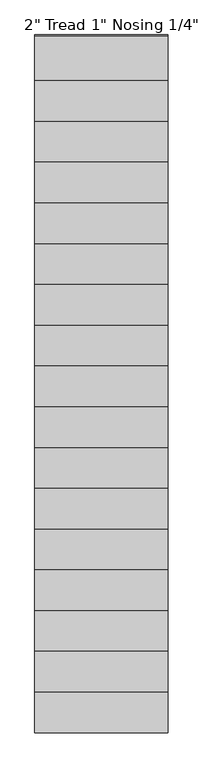
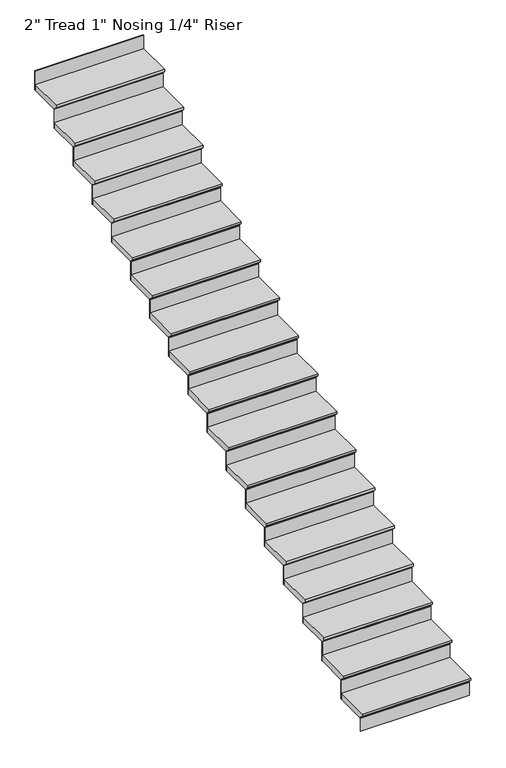
"""IFC4 building model written with IfcOpenShell, lengths in millimetres: stair flight geometry."""

from ifc_helpers import new_model, si_unit, frame, origin, place, context, project, spatial, polyline, outline, extrude, source, transform, mapped, element, save


def stair_flight_6f7ba89f(model_context):
    return source(origin(), model_context, "Body", "SweptSolid", [
        extrude(outline(polyline([(2020.7325341, 3522.1333333), (2325.5325341, 3522.1333333), (2325.5325341, 3471.3333333), (2046.1325341, 3471.3333333), (2046.1325341, 3477.6833333), (2020.7325341, 3503.0833333), (2020.7325341, 3522.1333333)])), frame((-5721.5875748, 0.0, 0.0), z_axis=(1.0, 0.0, 0.0), x_axis=(0.0, 1.0, 0.0)), (0.0, 0.0, 1.0), 914.4),
        extrude(outline(polyline([(-4807.1875748, 2052.4825341), (-4807.1875748, 2046.1325341), (-5721.5875748, 2046.1325341), (-5721.5875748, 2052.4825341), (-4807.1875748, 2052.4825341)])), frame((0.0, 0.0, 3352.8), z_axis=(0.0, 0.0, 1.0), x_axis=(1.0, 0.0, 0.0)), (0.0, 0.0, 1.0), 118.5333333),
        extrude(outline(polyline([(-4807.1875748, 2331.8825341), (-4807.1875748, 2325.5325341), (-5721.5875748, 2325.5325341), (-5721.5875748, 2331.8825341), (-4807.1875748, 2331.8825341)])), frame((0.0, 0.0, 3471.3333333), z_axis=(0.0, 0.0, 1.0), x_axis=(1.0, 0.0, 0.0)), (0.0, 0.0, 1.0), 169.3333333),
        extrude(outline(polyline([(2300.1325341, 3691.4666667), (2604.9325341, 3691.4666667), (2604.9325341, 3640.6666667), (2325.5325341, 3640.6666667), (2325.5325341, 3647.0166667), (2300.1325341, 3672.4166667), (2300.1325341, 3691.4666667)])), frame((-5721.5875748, 0.0, 0.0), z_axis=(1.0, 0.0, 0.0), x_axis=(0.0, 1.0, 0.0)), (0.0, 0.0, 1.0), 914.4),
        extrude(outline(polyline([(-4807.1875748, 2611.2825341), (-4807.1875748, 2604.9325341), (-5721.5875748, 2604.9325341), (-5721.5875748, 2611.2825341), (-4807.1875748, 2611.2825341)])), frame((0.0, 0.0, 3640.6666667), z_axis=(0.0, 0.0, 1.0), x_axis=(1.0, 0.0, 0.0)), (0.0, 0.0, 1.0), 169.3333333),
        extrude(outline(polyline([(2579.5325341, 3860.8), (2884.3325341, 3860.8), (2884.3325341, 3810.0), (2604.9325341, 3810.0), (2604.9325341, 3816.35), (2579.5325341, 3841.75), (2579.5325341, 3860.8)])), frame((-5721.5875748, 0.0, 0.0), z_axis=(1.0, 0.0, 0.0), x_axis=(0.0, 1.0, 0.0)), (0.0, 0.0, 1.0), 914.4),
        extrude(outline(polyline([(-4807.1875748, 2890.6825341), (-4807.1875748, 2884.3325341), (-5721.5875748, 2884.3325341), (-5721.5875748, 2890.6825341), (-4807.1875748, 2890.6825341)])), frame((0.0, 0.0, 3810.0), z_axis=(0.0, 0.0, 1.0), x_axis=(1.0, 0.0, 0.0)), (0.0, 0.0, 1.0), 169.3333333),
        extrude(outline(polyline([(2858.9325341, 4030.1333333), (3163.7325341, 4030.1333333), (3163.7325341, 3979.3333333), (2884.3325341, 3979.3333333), (2884.3325341, 3985.6833333), (2858.9325341, 4011.0833333), (2858.9325341, 4030.1333333)])), frame((-5721.5875748, 0.0, 0.0), z_axis=(1.0, 0.0, 0.0), x_axis=(0.0, 1.0, 0.0)), (0.0, 0.0, 1.0), 914.4),
        extrude(outline(polyline([(-4807.1875748, 3170.0825341), (-4807.1875748, 3163.7325341), (-5721.5875748, 3163.7325341), (-5721.5875748, 3170.0825341), (-4807.1875748, 3170.0825341)])), frame((0.0, 0.0, 3979.3333333), z_axis=(0.0, 0.0, 1.0), x_axis=(1.0, 0.0, 0.0)), (0.0, 0.0, 1.0), 169.3333333),
        extrude(outline(polyline([(3138.3325341, 4199.4666667), (3443.1325341, 4199.4666667), (3443.1325341, 4148.6666667), (3163.7325341, 4148.6666667), (3163.7325341, 4155.0166667), (3138.3325341, 4180.4166667), (3138.3325341, 4199.4666667)])), frame((-5721.5875748, 0.0, 0.0), z_axis=(1.0, 0.0, 0.0), x_axis=(0.0, 1.0, 0.0)), (0.0, 0.0, 1.0), 914.4),
        extrude(outline(polyline([(-4807.1875748, 3449.4825341), (-4807.1875748, 3443.1325341), (-5721.5875748, 3443.1325341), (-5721.5875748, 3449.4825341), (-4807.1875748, 3449.4825341)])), frame((0.0, 0.0, 4148.6666667), z_axis=(0.0, 0.0, 1.0), x_axis=(1.0, 0.0, 0.0)), (0.0, 0.0, 1.0), 169.3333333),
        extrude(outline(polyline([(3417.7325341, 4368.8), (3722.5325341, 4368.8), (3722.5325341, 4318.0), (3443.1325341, 4318.0), (3443.1325341, 4324.35), (3417.7325341, 4349.75), (3417.7325341, 4368.8)])), frame((-5721.5875748, 0.0, 0.0), z_axis=(1.0, 0.0, 0.0), x_axis=(0.0, 1.0, 0.0)), (0.0, 0.0, 1.0), 914.4),
        extrude(outline(polyline([(-4807.1875748, 3728.8825341), (-4807.1875748, 3722.5325341), (-5721.5875748, 3722.5325341), (-5721.5875748, 3728.8825341), (-4807.1875748, 3728.8825341)])), frame((0.0, 0.0, 4318.0), z_axis=(0.0, 0.0, 1.0), x_axis=(1.0, 0.0, 0.0)), (0.0, 0.0, 1.0), 169.3333333),
        extrude(outline(polyline([(3697.1325341, 4538.1333333), (4001.9325341, 4538.1333333), (4001.9325341, 4487.3333333), (3722.5325341, 4487.3333333), (3722.5325341, 4493.6833333), (3697.1325341, 4519.0833333), (3697.1325341, 4538.1333333)])), frame((-5721.5875748, 0.0, 0.0), z_axis=(1.0, 0.0, 0.0), x_axis=(0.0, 1.0, 0.0)), (0.0, 0.0, 1.0), 914.4),
        extrude(outline(polyline([(-4807.1875748, 4008.2825341), (-4807.1875748, 4001.9325341), (-5721.5875748, 4001.9325341), (-5721.5875748, 4008.2825341), (-4807.1875748, 4008.2825341)])), frame((0.0, 0.0, 4487.3333333), z_axis=(0.0, 0.0, 1.0), x_axis=(1.0, 0.0, 0.0)), (0.0, 0.0, 1.0), 169.3333333),
        extrude(outline(polyline([(3976.5325341, 4707.4666667), (4281.3325341, 4707.4666667), (4281.3325341, 4656.6666667), (4001.9325341, 4656.6666667), (4001.9325341, 4663.0166667), (3976.5325341, 4688.4166667), (3976.5325341, 4707.4666667)])), frame((-5721.5875748, 0.0, 0.0), z_axis=(1.0, 0.0, 0.0), x_axis=(0.0, 1.0, 0.0)), (0.0, 0.0, 1.0), 914.4),
        extrude(outline(polyline([(-4807.1875748, 4287.6825341), (-4807.1875748, 4281.3325341), (-5721.5875748, 4281.3325341), (-5721.5875748, 4287.6825341), (-4807.1875748, 4287.6825341)])), frame((0.0, 0.0, 4656.6666667), z_axis=(0.0, 0.0, 1.0), x_axis=(1.0, 0.0, 0.0)), (0.0, 0.0, 1.0), 169.3333333),
        extrude(outline(polyline([(4255.9325341, 4876.8), (4560.7325341, 4876.8), (4560.7325341, 4826.0), (4281.3325341, 4826.0), (4281.3325341, 4832.35), (4255.9325341, 4857.75), (4255.9325341, 4876.8)])), frame((-5721.5875748, 0.0, 0.0), z_axis=(1.0, 0.0, 0.0), x_axis=(0.0, 1.0, 0.0)), (0.0, 0.0, 1.0), 914.4),
        extrude(outline(polyline([(-4807.1875748, 4567.0825341), (-4807.1875748, 4560.7325341), (-5721.5875748, 4560.7325341), (-5721.5875748, 4567.0825341), (-4807.1875748, 4567.0825341)])), frame((0.0, 0.0, 4826.0), z_axis=(0.0, 0.0, 1.0), x_axis=(1.0, 0.0, 0.0)), (0.0, 0.0, 1.0), 169.3333333),
        extrude(outline(polyline([(4535.3325341, 5046.1333333), (4840.1325341, 5046.1333333), (4840.1325341, 4995.3333333), (4560.7325341, 4995.3333333), (4560.7325341, 5001.6833333), (4535.3325341, 5027.0833333), (4535.3325341, 5046.1333333)])), frame((-5721.5875748, 0.0, 0.0), z_axis=(1.0, 0.0, 0.0), x_axis=(0.0, 1.0, 0.0)), (0.0, 0.0, 1.0), 914.4),
        extrude(outline(polyline([(-4807.1875748, 4846.4825341), (-4807.1875748, 4840.1325341), (-5721.5875748, 4840.1325341), (-5721.5875748, 4846.4825341), (-4807.1875748, 4846.4825341)])), frame((0.0, 0.0, 4995.3333333), z_axis=(0.0, 0.0, 1.0), x_axis=(1.0, 0.0, 0.0)), (0.0, 0.0, 1.0), 169.3333333),
        extrude(outline(polyline([(4814.7325341, 5215.4666667), (5119.5325341, 5215.4666667), (5119.5325341, 5164.6666667), (4840.1325341, 5164.6666667), (4840.1325341, 5171.0166667), (4814.7325341, 5196.4166667), (4814.7325341, 5215.4666667)])), frame((-5721.5875748, 0.0, 0.0), z_axis=(1.0, 0.0, 0.0), x_axis=(0.0, 1.0, 0.0)), (0.0, 0.0, 1.0), 914.4),
        extrude(outline(polyline([(-4807.1875748, 5125.8825341), (-4807.1875748, 5119.5325341), (-5721.5875748, 5119.5325341), (-5721.5875748, 5125.8825341), (-4807.1875748, 5125.8825341)])), frame((0.0, 0.0, 5164.6666667), z_axis=(0.0, 0.0, 1.0), x_axis=(1.0, 0.0, 0.0)), (0.0, 0.0, 1.0), 169.3333333),
        extrude(outline(polyline([(5094.1325341, 5384.8), (5398.9325341, 5384.8), (5398.9325341, 5334.0), (5119.5325341, 5334.0), (5119.5325341, 5340.35), (5094.1325341, 5365.75), (5094.1325341, 5384.8)])), frame((-5721.5875748, 0.0, 0.0), z_axis=(1.0, 0.0, 0.0), x_axis=(0.0, 1.0, 0.0)), (0.0, 0.0, 1.0), 914.4),
        extrude(outline(polyline([(-4807.1875748, 5405.2825341), (-4807.1875748, 5398.9325341), (-5721.5875748, 5398.9325341), (-5721.5875748, 5405.2825341), (-4807.1875748, 5405.2825341)])), frame((0.0, 0.0, 5334.0), z_axis=(0.0, 0.0, 1.0), x_axis=(1.0, 0.0, 0.0)), (0.0, 0.0, 1.0), 169.3333333),
        extrude(outline(polyline([(5373.5325341, 5554.1333333), (5678.3325341, 5554.1333333), (5678.3325341, 5503.3333333), (5398.9325341, 5503.3333333), (5398.9325341, 5509.6833333), (5373.5325341, 5535.0833333), (5373.5325341, 5554.1333333)])), frame((-5721.5875748, 0.0, 0.0), z_axis=(1.0, 0.0, 0.0), x_axis=(0.0, 1.0, 0.0)), (0.0, 0.0, 1.0), 914.4),
        extrude(outline(polyline([(-4807.1875748, 5684.6825341), (-4807.1875748, 5678.3325341), (-5721.5875748, 5678.3325341), (-5721.5875748, 5684.6825341), (-4807.1875748, 5684.6825341)])), frame((0.0, 0.0, 5503.3333333), z_axis=(0.0, 0.0, 1.0), x_axis=(1.0, 0.0, 0.0)), (0.0, 0.0, 1.0), 169.3333333),
        extrude(outline(polyline([(5652.9325341, 5723.4666667), (5957.7325341, 5723.4666667), (5957.7325341, 5672.6666667), (5678.3325341, 5672.6666667), (5678.3325341, 5679.0166667), (5652.9325341, 5704.4166667), (5652.9325341, 5723.4666667)])), frame((-5721.5875748, 0.0, 0.0), z_axis=(1.0, 0.0, 0.0), x_axis=(0.0, 1.0, 0.0)), (0.0, 0.0, 1.0), 914.4),
        extrude(outline(polyline([(-4807.1875748, 5964.0825341), (-4807.1875748, 5957.7325341), (-5721.5875748, 5957.7325341), (-5721.5875748, 5964.0825341), (-4807.1875748, 5964.0825341)])), frame((0.0, 0.0, 5672.6666667), z_axis=(0.0, 0.0, 1.0), x_axis=(1.0, 0.0, 0.0)), (0.0, 0.0, 1.0), 169.3333333),
        extrude(outline(polyline([(5932.3325341, 5892.8), (6237.1325341, 5892.8), (6237.1325341, 5842.0), (5957.7325341, 5842.0), (5957.7325341, 5848.35), (5932.3325341, 5873.75), (5932.3325341, 5892.8)])), frame((-5721.5875748, 0.0, 0.0), z_axis=(1.0, 0.0, 0.0), x_axis=(0.0, 1.0, 0.0)), (0.0, 0.0, 1.0), 914.4),
        extrude(outline(polyline([(-4807.1875748, 6243.4825341), (-4807.1875748, 6237.1325341), (-5721.5875748, 6237.1325341), (-5721.5875748, 6243.4825341), (-4807.1875748, 6243.4825341)])), frame((0.0, 0.0, 5842.0), z_axis=(0.0, 0.0, 1.0), x_axis=(1.0, 0.0, 0.0)), (0.0, 0.0, 1.0), 169.3333333),
        extrude(outline(polyline([(6211.7325341, 6062.1333333), (6516.5325341, 6062.1333333), (6516.5325341, 6011.3333333), (6237.1325341, 6011.3333333), (6237.1325341, 6017.6833333), (6211.7325341, 6043.0833333), (6211.7325341, 6062.1333333)])), frame((-5721.5875748, 0.0, 0.0), z_axis=(1.0, 0.0, 0.0), x_axis=(0.0, 1.0, 0.0)), (0.0, 0.0, 1.0), 914.4),
        extrude(outline(polyline([(-4807.1875748, 6522.8825341), (-4807.1875748, 6516.5325341), (-5721.5875748, 6516.5325341), (-5721.5875748, 6522.8825341), (-4807.1875748, 6522.8825341)])), frame((0.0, 0.0, 6011.3333333), z_axis=(0.0, 0.0, 1.0), x_axis=(1.0, 0.0, 0.0)), (0.0, 0.0, 1.0), 169.3333333),
        extrude(outline(polyline([(-4807.1875748, 6802.2825341), (-4807.1875748, 6795.9325341), (-5721.5875748, 6795.9325341), (-5721.5875748, 6802.2825341), (-4807.1875748, 6802.2825341)])), frame((0.0, 0.0, 6180.6666667), z_axis=(0.0, 0.0, 1.0), x_axis=(1.0, 0.0, 0.0)), (0.0, 0.0, 1.0), 169.3333333),
        extrude(outline(polyline([(6491.1325341, 6231.4666667), (6795.9325341, 6231.4666667), (6795.9325341, 6180.6666667), (6516.5325341, 6180.6666667), (6516.5325341, 6187.0166667), (6491.1325341, 6212.4166667), (6491.1325341, 6231.4666667)])), frame((-5721.5875748, 0.0, 0.0), z_axis=(1.0, 0.0, 0.0), x_axis=(0.0, 1.0, 0.0)), (0.0, 0.0, 1.0), 914.4),
    ])


if __name__ == "__main__":
    model = new_model("IFC4")
    model_context = context("Model", 3, world=origin())
    ifc_project = project(units=[si_unit("LENGTHUNIT", "METRE", prefix="MILLI")], contexts=[model_context])
    site = spatial("IfcSite", under=ifc_project)
    building = spatial("IfcBuilding", under=site)
    placement = place(None, origin())
    stair_flight_shape = stair_flight_6f7ba89f(model_context)
    element("IfcStairFlight", 1, ObjectType="2\" Tread 1\" Nosing 1/4\" Riser", at=placement, inside=building, context=model_context, shape_type="MappedRepresentation", body=[
        mapped(stair_flight_shape, transform((0.0, 0.0, 0.0), x_axis=(1.0, 0.0, 0.0), y_axis=(0.0, 1.0, 0.0), z_axis=(0.0, 0.0, 1.0))),
    ])
    save(model, "model.ifc")
